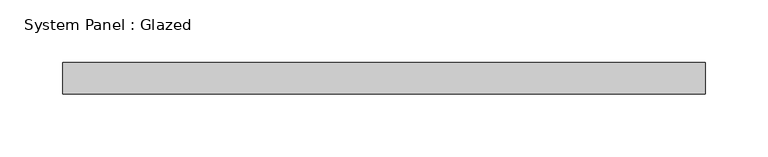
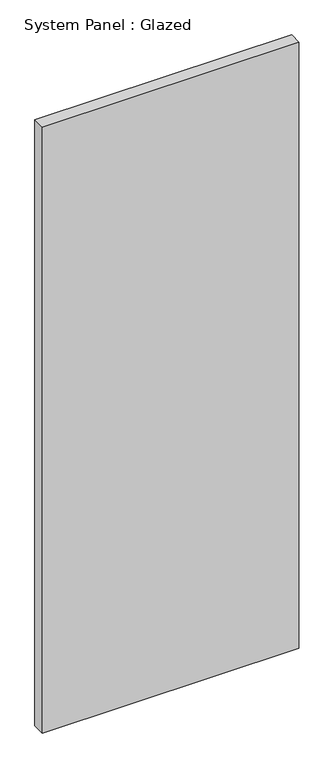
"""IFC4 building model written with IfcOpenShell, lengths in millimetres: plate geometry, System Panel : Glazed."""

from ifc_helpers import new_model, si_unit, origin, origin_with_axes, place, context, project, spatial, polyline, outline, extrude, source, transform, mapped, element, save


def system_panel_glazed_e08f8b61(model_context):
    return source(origin(), model_context, "Body", "SweptSolid", [
        extrude(outline(polyline([(257.175, 19.05), (-257.175, 19.05), (-257.175, 44.45), (257.175, 44.45), (257.175, 19.05)])), origin_with_axes(), (0.0, 0.0, 1.0), 1283.3945466),
    ])


if __name__ == "__main__":
    model = new_model("IFC4")
    model_context = context("Model", 3, world=origin())
    ifc_project = project(units=[si_unit("LENGTHUNIT", "METRE", prefix="MILLI")], contexts=[model_context])
    site = spatial("IfcSite", under=ifc_project)
    building = spatial("IfcBuilding", under=site)
    placement = place(None, origin())
    system_panel_glazed_shape = system_panel_glazed_e08f8b61(model_context)
    element("IfcPlate", 1, ObjectType="System Panel : Glazed", at=placement, inside=building, context=model_context, shape_type="MappedRepresentation", body=[
        mapped(system_panel_glazed_shape, transform((0.0, 0.0, 0.0), x_axis=(1.0, 0.0, 0.0), y_axis=(0.0, 1.0, 0.0), z_axis=(0.0, 0.0, 1.0))),
    ])
    save(model, "model.ifc")

# Revit data of these elements
# Type "System Panel : Glazed"
#   Construction Type Id = "GSP4R"
#   Analytic Construction = "1/8 in Pilkington single glazing"
#   Visual Light Transmittance = 0.9
#   Solar Heat Gain Coefficient = 0.86
#   Heat Transfer Coefficient (U) = 1.18115 BTU/(h·ft²·°F)
#   Define Thermal Properties by = 1
# Element 1 (IfcPlate, "System Panel : Glazed")
#   Materials on its faces: "Glass"
# Materials
#   "Glass": class "Glass", colour RGB 0 128 192, transparency 0.75, Description = "Soda Lime Glass", Cost = 0
